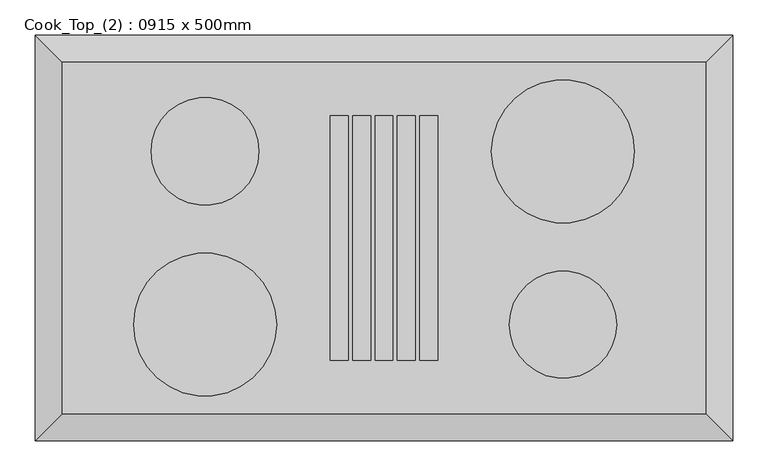
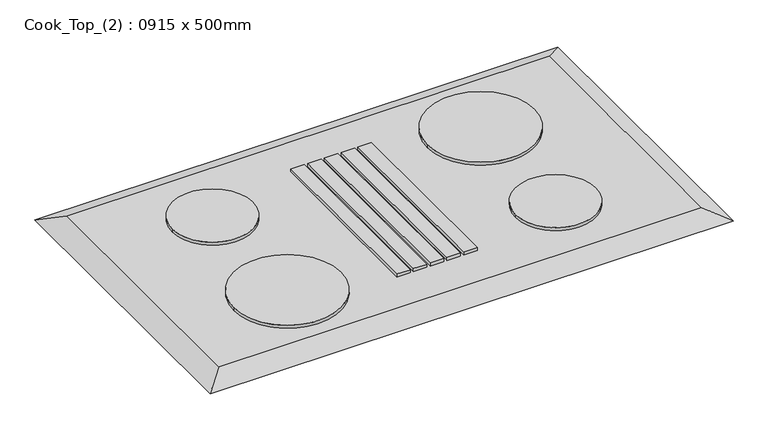
"""IFC4 building model written with IfcOpenShell, lengths in millimetres: proxy geometry, Cook_Top_(2) : 0915 x 500mm."""

from ifc_helpers import new_model, si_unit, point, frame, frame_2d, origin, place, context, project, spatial, polyline, circle_curve, trimmed, segment, composite_curve, outline, extrude, faceted_brep, source, transform, mapped, element, save


def cook_top_2_0915_x_500mm_892363c5(model_context):
    return source(origin(), model_context, "Body", "SolidModel", [
        faceted_brep([(457.5, 250.0, 918.0), (-457.5, 250.0, 918.0), (-457.5, -250.0, 918.0), (457.5, -250.0, 918.0), (495.6, 288.1, 900.0), (495.6, -288.1, 900.0), (-495.6, -288.1, 900.0), (-495.6, 288.1, 900.0)], [[[0, 1, 2, 3]], [[4, 5, 6, 7]], [[4, 7, 1, 0]], [[7, 6, 2, 1]], [[6, 5, 3, 2]], [[5, 4, 0, 3]]]),
        extrude(outline(composite_curve([segment(trimmed(circle_curve(frame_2d((-254.3, 123.0)), 76.5869489), [point((-177.7130511, 123.0))], [point((-330.8869489, 123.0))], False, "CARTESIAN"), True, "CONTINUOUS"), segment(trimmed(circle_curve(frame_2d((-254.3, 123.0)), 76.5869489), [point((-330.8869489, 123.0))], [point((-177.7130511, 123.0))], False, "CARTESIAN"), True, "CONTINUOUS")], self_intersect=False)), frame((0.0, 0.0, 918.0), z_axis=(0.0, 0.0, 1.0), x_axis=(1.0, 0.0, 0.0)), (0.0, 0.0, 1.0), 6.35),
        extrude(outline(composite_curve([segment(trimmed(circle_curve(frame_2d((254.3, 123.0)), 101.6), [point((355.9, 123.0))], [point((152.7, 123.0))], False, "CARTESIAN"), True, "CONTINUOUS"), segment(trimmed(circle_curve(frame_2d((254.3, 123.0)), 101.6), [point((152.7, 123.0))], [point((355.9, 123.0))], False, "CARTESIAN"), True, "CONTINUOUS")], self_intersect=False)), frame((0.0, 0.0, 918.0), z_axis=(0.0, 0.0, 1.0), x_axis=(1.0, 0.0, 0.0)), (0.0, 0.0, 1.0), 6.35),
        extrude(outline(composite_curve([segment(trimmed(circle_curve(frame_2d((254.3, -123.0)), 76.2), [point((330.5, -123.0))], [point((178.1, -123.0))], False, "CARTESIAN"), True, "CONTINUOUS"), segment(trimmed(circle_curve(frame_2d((254.3, -123.0)), 76.2), [point((178.1, -123.0))], [point((330.5, -123.0))], False, "CARTESIAN"), True, "CONTINUOUS")], self_intersect=False)), frame((0.0, 0.0, 918.0), z_axis=(0.0, 0.0, 1.0), x_axis=(1.0, 0.0, 0.0)), (0.0, 0.0, 1.0), 6.35),
        extrude(outline(polyline([(-50.8, 173.8), (-50.8, -173.8), (-76.2, -173.8), (-76.2, 173.8), (-50.8, 173.8)])), frame((0.0, 0.0, 918.0), z_axis=(0.0, 0.0, 1.0), x_axis=(1.0, 0.0, 0.0)), (0.0, 0.0, 1.0), 6.35),
        extrude(outline(polyline([(-19.05, 173.8), (-19.05, -173.8), (-44.45, -173.8), (-44.45, 173.8), (-19.05, 173.8)])), frame((0.0, 0.0, 918.0), z_axis=(0.0, 0.0, 1.0), x_axis=(1.0, 0.0, 0.0)), (0.0, 0.0, 1.0), 6.35),
        extrude(outline(polyline([(12.7, 173.8), (12.7, -173.8), (-12.7, -173.8), (-12.7, 173.8), (12.7, 173.8)])), frame((0.0, 0.0, 918.0), z_axis=(0.0, 0.0, 1.0), x_axis=(1.0, 0.0, 0.0)), (0.0, 0.0, 1.0), 6.35),
        extrude(outline(polyline([(44.45, 173.8), (44.45, -173.8), (19.05, -173.8), (19.05, 173.8), (44.45, 173.8)])), frame((0.0, 0.0, 918.0), z_axis=(0.0, 0.0, 1.0), x_axis=(1.0, 0.0, 0.0)), (0.0, 0.0, 1.0), 6.35),
        extrude(outline(polyline([(76.2, 173.8), (76.2, -173.8), (50.8, -173.8), (50.8, 173.8), (76.2, 173.8)])), frame((0.0, 0.0, 918.0), z_axis=(0.0, 0.0, 1.0), x_axis=(1.0, 0.0, 0.0)), (0.0, 0.0, 1.0), 6.35),
        extrude(outline(composite_curve([segment(trimmed(circle_curve(frame_2d((-254.3, -123.0)), 101.6), [point((-152.7, -123.0))], [point((-355.9, -123.0))], False, "CARTESIAN"), True, "CONTINUOUS"), segment(trimmed(circle_curve(frame_2d((-254.3, -123.0)), 101.6), [point((-355.9, -123.0))], [point((-152.7, -123.0))], False, "CARTESIAN"), True, "CONTINUOUS")], self_intersect=False)), frame((0.0, 0.0, 918.0), z_axis=(0.0, 0.0, 1.0), x_axis=(1.0, 0.0, 0.0)), (0.0, 0.0, 1.0), 6.35),
    ])


if __name__ == "__main__":
    model = new_model("IFC4")
    model_context = context("Model", 3, world=origin())
    ifc_project = project(units=[si_unit("LENGTHUNIT", "METRE", prefix="MILLI")], contexts=[model_context])
    site = spatial("IfcSite", under=ifc_project)
    building = spatial("IfcBuilding", under=site)
    placement = place(None, origin())
    cook_top_2_0915_x_500mm_shape = cook_top_2_0915_x_500mm_892363c5(model_context)
    element("IfcBuildingElementProxy", 1, Name="Cook_Top_(2) : 0915 x 500mm", ObjectType="Cook_Top_(2) : 0915 x 500mm", at=placement, inside=building, context=model_context, shape_type="MappedRepresentation", body=[
        mapped(cook_top_2_0915_x_500mm_shape, transform((0.0, 0.0, 0.0), x_axis=(1.0, 0.0, 0.0), y_axis=(0.0, 1.0, 0.0), z_axis=(0.0, 0.0, 1.0))),
    ])
    save(model, "model.ifc")

# Revit data of these elements
# Type "Cook_Top_(2) : 0915 x 500mm"
#   Keynote = "N"
#   Depth = 1.64042 ft
#   Width = 3.001969 ft
#   Material Burner = Metal - Chrome
#   Material Cooktop = Metal - Steel, Polished
#   Default Elevation = 0
# Element 1 (IfcBuildingElementProxy, "Cook_Top_(2) : 0915 x 500mm")
#   Materials on its faces: "Metal - Chrome", "Metal - Steel, Polished"
# Materials
#   "Metal - Chrome": colour RGB 247 247 247, transparency 0
#   "Metal - Steel, Polished": colour RGB 247 247 247, transparency 0
